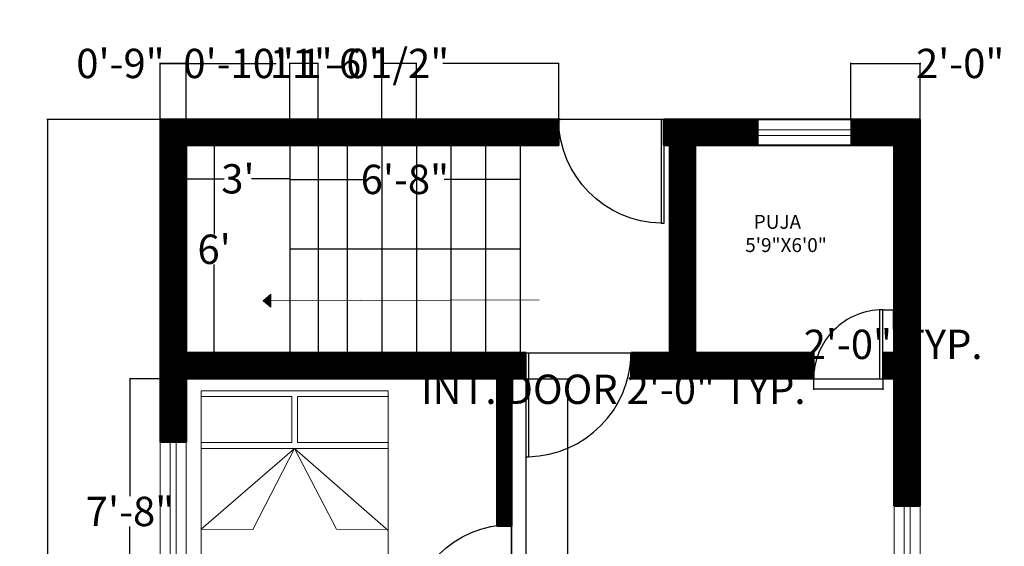
# Model space of a CAD drawing. Units: inches. Extents: x 254 to 1358, y 67 to 796.
# Tile 2 of 3: x 254 to 596, y 313 to 496. Entities that reach past the tile are written whole.
import ezdxf

# ---------------------------------------------------------------- set-up
doc = ezdxf.new("R2010")
doc.units = ezdxf.units.IN
doc.header["$MEASUREMENT"] = 0
for name, color, linetype, lineweight in [('A-ANNO-DIMS', 2, 'Continuous', 18), ('A-ANNO-SYMB', 7, 'Continuous', 18), ('A-AREA-IDEN', 7, 'Continuous', 18), ('A-FLOR-STRS', 7, 'Continuous', 25), ('A-FURN', 8, 'Continuous', 18), ('A-GLAZ', 160, 'Continuous', 18), ('A-WALL', 7, 'Continuous', 40), ('doors', 8, 'Continuous', 25)]:
    doc.layers.add(name, color=color, linetype=linetype, lineweight=lineweight)
doc.layers.add('A-ANNO-SYMB-PATT', color=251, linetype='Continuous', lineweight=13, true_color=0x636466)
doc.layers.add('A-WALL-PATT', color=251, linetype='Continuous', lineweight=13, true_color=0x636466)
doc.styles.get("Standard").update_dxf_attribs({"font": 'arial.ttf'})
doc.dimstyles.get("Standard").update_dxf_attribs({"dimtxt": 10.18, "dimasz": 0.18, "dimexe": 0.18, "dimexo": 0.0625, "dimgap": 0.09, "dimtad": 0, "dimtih": 1, "dimtoh": 1, "dimdec": 0, "dimzin": 0, "dimdsep": 46, "dimlunit": 3, "dimtxsty": 'Standard', "dimcen": 0.09, "dimadec": 0, "dimazin": 0, "dimtfac": 1, "dimtdec": 0, "dimtofl": 0, "dimtmove": 0, "dimatfit": 3, "dimfxl": 1, "dimtolj": 1, "dimtzin": 0, "dimarcsym": 0})

# ---------------------------------------------------------------- blocks, each defined once
blk = doc.blocks.new('*D1')
at = {"layer": 'A-ANNO-DIMS', "color": 0, "lineweight": -2, "transparency": 16777216}
for p, q in [((311.39, 452.48), (311.39, 440.81)), ((347.39, 452.48), (347.39, 440.81)), ((311.57, 440.99), (324.62, 440.99)), ((347.21, 440.99), (334.16, 440.99))]:
    blk.add_line(p, q, dxfattribs=at)
at = {"layer": 'A-ANNO-DIMS', "color": 0, "transparency": 16777216}
for points in [[(311.57, 441.02), (311.57, 440.96), (311.39, 440.99)], [(347.21, 441.02), (347.21, 440.96), (347.39, 440.99)]]:
    blk.add_solid(points, dxfattribs=at)
at = {"layer": 'Defpoints', "color": 0, "transparency": 16777216}
for p in [(311.39, 452.54), (347.39, 452.54), (347.39, 440.99)]:
    blk.add_point(p, dxfattribs=at)
at = {"layer": 'A-ANNO-DIMS', "color": 0, "transparency": 16777216, "insert": (329.39, 440.99), "char_height": 10.18, "attachment_point": 5}
blk.add_mtext("\\A1;3'", dxfattribs=at)
blk = doc.blocks.new('*D2')
at = {"layer": 'A-ANNO-DIMS', "color": 0, "lineweight": -2, "transparency": 16777216}
for p, q in [((347.39, 452.48), (347.39, 440.61)), ((427.39, 452.48), (427.39, 440.61)), ((347.57, 440.79), (373.74, 440.79)), ((427.21, 440.79), (401.04, 440.79))]:
    blk.add_line(p, q, dxfattribs=at)
at = {"layer": 'A-ANNO-DIMS', "color": 0, "transparency": 16777216}
for points in [[(347.57, 440.82), (347.57, 440.76), (347.39, 440.79)], [(427.21, 440.82), (427.21, 440.76), (427.39, 440.79)]]:
    blk.add_solid(points, dxfattribs=at)
at = {"layer": 'Defpoints', "color": 0, "transparency": 16777216}
for p in [(347.39, 452.54), (427.39, 452.54), (427.39, 440.79)]:
    blk.add_point(p, dxfattribs=at)
at = {"layer": 'A-ANNO-DIMS', "color": 0, "transparency": 16777216, "insert": (387.39, 440.79), "char_height": 10.18, "attachment_point": 5}
blk.add_mtext('\\A1;6\'-8"', dxfattribs=at)
blk = doc.blocks.new('*D3')
at = {"layer": 'A-ANNO-DIMS', "color": 0, "lineweight": -2, "transparency": 16777216}
for p, q in [((311.46, 452.54), (321.31, 452.54)), ((321.13, 452.36), (321.13, 421.83)), ((321.13, 380.72), (321.13, 411.26)), ((311.46, 380.54), (321.31, 380.54))]:
    blk.add_line(p, q, dxfattribs=at)
at = {"layer": 'A-ANNO-DIMS', "color": 0, "transparency": 16777216}
for points in [[(321.1, 452.36), (321.16, 452.36), (321.13, 452.54)], [(321.1, 380.72), (321.16, 380.72), (321.13, 380.54)]]:
    blk.add_solid(points, dxfattribs=at)
at = {"layer": 'Defpoints', "color": 0, "transparency": 16777216}
for p in [(311.39, 452.54), (311.39, 380.54), (321.13, 380.54)]:
    blk.add_point(p, dxfattribs=at)
at = {"layer": 'A-ANNO-DIMS', "color": 0, "transparency": 16777216, "insert": (321.13, 416.54), "char_height": 10.18, "attachment_point": 5}
blk.add_mtext("\\A1;6'", dxfattribs=at)
blk = doc.blocks.new('*D4')
at = {"layer": 'A-ANNO-DIMS', "color": 0, "lineweight": -2, "transparency": 16777216}
for p, q in [((302.33, 461.54), (263.04, 461.54)), ((263.22, 461.36), (263.22, 286.83)), ((263.22, 101.72), (263.22, 276.25)), ((302.33, 101.54), (263.04, 101.54))]:
    blk.add_line(p, q, dxfattribs=at)
at = {"layer": 'A-ANNO-DIMS', "color": 0, "transparency": 16777216}
for points in [[(263.19, 461.36), (263.25, 461.36), (263.22, 461.54)], [(263.19, 101.72), (263.25, 101.72), (263.22, 101.54)]]:
    blk.add_solid(points, dxfattribs=at)
at = {"layer": 'Defpoints', "color": 0, "transparency": 16777216}
for p in [(302.39, 461.54), (263.22, 101.54), (302.39, 101.54)]:
    blk.add_point(p, dxfattribs=at)
at = {"layer": 'A-ANNO-DIMS', "color": 0, "transparency": 16777216, "insert": (263.22, 281.54), "char_height": 10.18, "attachment_point": 5}
blk.add_mtext("\\A1;30'", dxfattribs=at)
blk = doc.blocks.new('WIN-48')
for p, q in [((9, 48), (0, 48)), ((0, 48), (0, 0)), ((3.5, 48), (3.5, 0)), ((5.5, 48), (5.5, 0)), ((5.5, 48), (5.5, 0)), ((5.5, 48), (5.5, 0)), ((5.5, 48), (5.5, 0)), ((9, 48), (9, 0)), ((9, 0), (0, 0))]:
    blk.add_line(p, q)
blk = doc.blocks.new('WIN-32')
for p, q in [((0, 0), (0, 9)), ((32.11, 9), (0, 9)), ((32.11, 0), (32.11, 9)), ((32.11, 5.5), (0, 5.5)), ((32.11, 3.5), (0, 3.5)), ((32.11, 3.5), (0, 3.5)), ((32.11, 3.5), (0, 3.5)), ((32.11, 3.5), (0, 3.5)), ((32.11, 0), (0, 0))]:
    blk.add_line(p, q)
blk = doc.blocks.new('DOOR-SWING-36')
for p, q in [((0, 0), (-36, 0)), ((-36, 0), (-36, -1)), ((0, 0), (0, -36.57)), ((0, -1), (-36, -1))]:
    blk.add_line(p, q)
blk.add_arc((0.31, -0.26), 36.31, 181.1696, 269.5155)
blk = doc.blocks.new('DOOR-SWING-24-INT')
for p, q in [((24, 0), (0, 0)), ((0, 0), (0, -24)), ((1, 0), (1, -24))]:
    blk.add_line(p, q)
blk.add_arc((0.03, -0.01), 23.97, 269.9169, 0.0334)
blk = doc.blocks.new('BED-DOUBLE')
for p, q in [((65, 72), (0, 72)), ((0, 72), (0, 0)), ((65, 0), (65, 72)), ((0, 48.04), (18, 48.19)), ((32.5, 20), (0, 48.04)), ((32.5, 20), (18, 48.19)), ((32.5, 20), (65, 48.44)), ((47, 48.04), (32.5, 20)), ((47, 48.04), (65, 48.19)), ((0, 20), (65, 20)), ((0, 18), (31.5, 18)), ((31.5, 18), (31.5, 2)), ((33.5, 18), (33.5, 2)), ((33.5, 18), (65, 18)), ((0, 2), (31.5, 2)), ((0, 0), (65, 0)), ((33.5, 2), (65, 2))]:
    blk.add_line(p, q)
blk = doc.blocks.new('*D28')
at = {"layer": 'A-ANNO-DIMS', "color": 0, "lineweight": -2, "transparency": 16777216}
for p, q in [((529.39, 371.48), (529.39, 367.76)), ((553.39, 371.48), (553.39, 367.76)), ((529.39, 367.94), (529.21, 367.94)), ((553.21, 367.94), (529.57, 367.94))]:
    blk.add_line(p, q, dxfattribs=at)
at = {"layer": 'A-ANNO-DIMS', "color": 0, "transparency": 16777216}
for points in [[(529.57, 367.97), (529.57, 367.91), (529.39, 367.94)], [(553.21, 367.97), (553.21, 367.91), (553.39, 367.94)]]:
    blk.add_solid(points, dxfattribs=at)
at = {"layer": 'Defpoints', "color": 0, "transparency": 16777216}
for p in [(529.39, 371.54), (553.39, 371.54), (529.39, 367.94)]:
    blk.add_point(p, dxfattribs=at)
at = {"layer": 'A-ANNO-DIMS', "color": 0, "transparency": 16777216, "insert": (459.75, 367.94), "char_height": 10.18, "attachment_point": 5}
blk.add_mtext('\\A1;INT. DOOR 2\'-0" TYP.', dxfattribs=at)
blk = doc.blocks.new('*D29')
at = {"layer": 'A-ANNO-DIMS', "color": 0, "lineweight": -2, "transparency": 16777216}
for p, q in [((553.46, 395.54), (557.17, 395.54)), ((556.99, 395.36), (556.99, 388.83)), ((556.99, 371.72), (556.99, 378.26)), ((553.46, 371.54), (557.17, 371.54))]:
    blk.add_line(p, q, dxfattribs=at)
at = {"layer": 'A-ANNO-DIMS', "color": 0, "transparency": 16777216}
for points in [[(556.96, 395.36), (557.02, 395.36), (556.99, 395.54)], [(556.96, 371.72), (557.02, 371.72), (556.99, 371.54)]]:
    blk.add_solid(points, dxfattribs=at)
at = {"layer": 'Defpoints', "color": 0, "transparency": 16777216}
for p in [(553.39, 395.54), (553.39, 371.54), (556.99, 371.54)]:
    blk.add_point(p, dxfattribs=at)
at = {"layer": 'A-ANNO-DIMS', "color": 0, "transparency": 16777216, "insert": (556.99, 383.54), "char_height": 10.18, "attachment_point": 5}
blk.add_mtext('\\A1;2\'-0" TYP.', dxfattribs=at)
blk = doc.blocks.new('*D41')
at = {"layer": 'A-ANNO-DIMS', "color": 0, "lineweight": -2, "transparency": 16777216}
for p, q in [((302.39, 461.61), (302.39, 481.21)), ((302.57, 481.03), (342.65, 481.03)), ((440.64, 481.03), (400.56, 481.03)), ((440.82, 461.6), (440.82, 481.21))]:
    blk.add_line(p, q, dxfattribs=at)
at = {"layer": 'A-ANNO-DIMS', "color": 0, "transparency": 16777216}
for points in [[(302.57, 481.06), (302.57, 481), (302.39, 481.03)], [(440.64, 481.06), (440.64, 481), (440.82, 481.03)]]:
    blk.add_solid(points, dxfattribs=at)
at = {"layer": 'Defpoints', "color": 0, "transparency": 16777216}
for p in [(440.82, 481.03), (302.39, 461.54), (440.82, 461.54)]:
    blk.add_point(p, dxfattribs=at)
at = {"layer": 'A-ANNO-DIMS', "color": 0, "transparency": 16777216, "insert": (371.61, 481.03), "char_height": 10.18, "attachment_point": 5}
blk.add_mtext('\\A1;11\'-6 1/2"', dxfattribs=at)
blk = doc.blocks.new('*D42')
at = {"layer": 'A-ANNO-DIMS', "color": 0, "lineweight": -2, "transparency": 16777216}
for p, q in [((542.27, 461.61), (542.27, 481.21)), ((542.45, 481.03), (566.21, 481.03)), ((566.39, 461.61), (566.39, 481.21)), ((566.39, 481.03), (566.57, 481.03))]:
    blk.add_line(p, q, dxfattribs=at)
at = {"layer": 'A-ANNO-DIMS', "color": 0, "transparency": 16777216}
for points in [[(542.45, 481.06), (542.45, 481), (542.27, 481.03)], [(566.21, 481.06), (566.21, 481), (566.39, 481.03)]]:
    blk.add_solid(points, dxfattribs=at)
at = {"layer": 'Defpoints', "color": 0, "transparency": 16777216}
for p in [(566.39, 481.03), (542.27, 461.54), (566.39, 461.54)]:
    blk.add_point(p, dxfattribs=at)
at = {"layer": 'A-ANNO-DIMS', "color": 0, "transparency": 16777216, "insert": (580.28, 481.03), "char_height": 10.18, "attachment_point": 5}
blk.add_mtext('\\A1;2\'-0"', dxfattribs=at)
blk = doc.blocks.new('*D45')
at = {"layer": 'A-ANNO-DIMS', "color": 0, "lineweight": -2, "transparency": 16777216}
for p, q in [((302.39, 481.03), (302.21, 481.03)), ((302.39, 461.61), (302.39, 481.21)), ((311.21, 481.03), (302.57, 481.03)), ((311.39, 452.61), (311.39, 481.21))]:
    blk.add_line(p, q, dxfattribs=at)
at = {"layer": 'A-ANNO-DIMS', "color": 0, "transparency": 16777216}
for points in [[(302.57, 481.06), (302.57, 481), (302.39, 481.03)], [(311.21, 481.06), (311.21, 481), (311.39, 481.03)]]:
    blk.add_solid(points, dxfattribs=at)
at = {"layer": 'Defpoints', "color": 0, "transparency": 16777216}
for p in [(302.39, 481.03), (302.39, 461.54), (311.39, 452.54)]:
    blk.add_point(p, dxfattribs=at)
at = {"layer": 'A-ANNO-DIMS', "color": 0, "transparency": 16777216, "insert": (288.59, 481.03), "char_height": 10.18, "attachment_point": 5}
blk.add_mtext('\\A1;0\'-9"', dxfattribs=at)
blk = doc.blocks.new('*D47')
at = {"layer": 'A-ANNO-DIMS', "color": 0, "lineweight": -2, "transparency": 16777216}
for p, q in [((311.33, 371.54), (291.72, 371.54)), ((291.9, 371.36), (291.9, 330.83)), ((291.9, 279.72), (291.9, 320.26)), ((311.33, 279.54), (291.72, 279.54))]:
    blk.add_line(p, q, dxfattribs=at)
at = {"layer": 'A-ANNO-DIMS', "color": 0, "transparency": 16777216}
for points in [[(291.87, 371.36), (291.93, 371.36), (291.9, 371.54)], [(291.87, 279.72), (291.93, 279.72), (291.9, 279.54)]]:
    blk.add_solid(points, dxfattribs=at)
at = {"layer": 'Defpoints', "color": 0, "transparency": 16777216}
for p in [(291.9, 371.54), (311.39, 371.54), (311.39, 279.54)]:
    blk.add_point(p, dxfattribs=at)
at = {"layer": 'A-ANNO-DIMS', "color": 0, "transparency": 16777216, "insert": (291.9, 325.54), "char_height": 10.18, "attachment_point": 5}
blk.add_mtext('\\A1;7\'-8"', dxfattribs=at)
blk = doc.blocks.new('*D49')
at = {"layer": 'A-ANNO-DIMS', "color": 0, "lineweight": -2, "transparency": 16777216}
for p, q in [((424.46, 371.54), (444.06, 371.54)), ((443.88, 371.36), (443.88, 308.74)), ((443.88, 235.72), (443.88, 298.34)), ((424.46, 235.54), (444.06, 235.54))]:
    blk.add_line(p, q, dxfattribs=at)
at = {"layer": 'A-ANNO-DIMS', "color": 0, "transparency": 16777216}
for points in [[(443.85, 371.36), (443.91, 371.36), (443.88, 371.54)], [(443.85, 235.72), (443.91, 235.72), (443.88, 235.54)]]:
    blk.add_solid(points, dxfattribs=at)
at = {"layer": 'Defpoints', "color": 0, "transparency": 16777216}
for p in [(424.39, 371.54), (424.39, 235.54), (443.88, 235.54)]:
    blk.add_point(p, dxfattribs=at)
at = {"layer": 'A-ANNO-DIMS', "color": 0, "transparency": 16777216, "insert": (443.88, 303.54), "char_height": 10.18, "attachment_point": 5}
blk.add_mtext('\\A1;11\'-4"', dxfattribs=at)
blk = doc.blocks.new('*D54')
at = {"layer": 'A-ANNO-DIMS', "color": 0, "lineweight": -2, "transparency": 16777216}
for p, q in [((347.39, 481.03), (347.21, 481.03)), ((347.39, 452.61), (347.39, 481.21)), ((357.12, 481.03), (347.57, 481.03)), ((357.3, 452.61), (357.3, 481.21))]:
    blk.add_line(p, q, dxfattribs=at)
at = {"layer": 'A-ANNO-DIMS', "color": 0, "transparency": 16777216}
for points in [[(347.57, 481.06), (347.57, 481), (347.39, 481.03)], [(357.12, 481.06), (357.12, 481), (357.3, 481.03)]]:
    blk.add_solid(points, dxfattribs=at)
at = {"layer": 'Defpoints', "color": 0, "transparency": 16777216}
for p in [(347.39, 481.03), (347.39, 452.54), (357.3, 452.54)]:
    blk.add_point(p, dxfattribs=at)
at = {"layer": 'A-ANNO-DIMS', "color": 0, "transparency": 16777216, "insert": (329.64, 481.03), "char_height": 10.18, "attachment_point": 5}
blk.add_mtext('\\A1;0\'-10"', dxfattribs=at)
blk = doc.blocks.new('*D55')
at = {"layer": 'A-ANNO-DIMS', "color": 0, "lineweight": -2, "transparency": 16777216}
for p, q in [((379.39, 481.03), (379.21, 481.03)), ((379.39, 452.61), (379.39, 481.21)), ((391.21, 481.03), (379.57, 481.03)), ((391.39, 452.61), (391.39, 481.21))]:
    blk.add_line(p, q, dxfattribs=at)
at = {"layer": 'A-ANNO-DIMS', "color": 0, "transparency": 16777216}
for points in [[(379.57, 481.06), (379.57, 481), (379.39, 481.03)], [(391.21, 481.06), (391.21, 481), (391.39, 481.03)]]:
    blk.add_solid(points, dxfattribs=at)
at = {"layer": 'Defpoints', "color": 0, "transparency": 16777216}
for p in [(379.39, 481.03), (379.39, 452.54), (391.39, 452.54)]:
    blk.add_point(p, dxfattribs=at)
at = {"layer": 'A-ANNO-DIMS', "color": 0, "transparency": 16777216, "insert": (366.07, 481.03), "char_height": 10.18, "attachment_point": 5}
blk.add_mtext('\\A1;1\'-0"', dxfattribs=at)
blk = doc.blocks.new('*D56')
at = {"layer": 'A-ANNO-DIMS', "color": 0, "lineweight": -2, "transparency": 16777216}
for p, q in [((429.39, 380.48), (429.39, 81.87)), ((424.39, 371.48), (424.39, 81.87)), ((424.57, 82.05), (429.21, 82.05)), ((429.39, 82.05), (429.57, 82.05))]:
    blk.add_line(p, q, dxfattribs=at)
at = {"layer": 'A-ANNO-DIMS', "color": 0, "transparency": 16777216}
for points in [[(424.57, 82.08), (424.57, 82.02), (424.39, 82.05)], [(429.21, 82.08), (429.21, 82.02), (429.39, 82.05)]]:
    blk.add_solid(points, dxfattribs=at)
at = {"layer": 'Defpoints', "color": 0, "transparency": 16777216}
for p in [(429.39, 380.54), (424.39, 371.54), (429.39, 82.05)]:
    blk.add_point(p, dxfattribs=at)
at = {"layer": 'A-ANNO-DIMS', "color": 0, "transparency": 16777216, "insert": (443.19, 82.05), "char_height": 10.18, "attachment_point": 5}
blk.add_mtext('\\A1;0\'-5"', dxfattribs=at)

msp = doc.modelspace()

# ---------------------------------------------------------------- hatches: boundary and pattern name
at = {"layer": 'A-ANNO-SYMB-PATT'}
h = msp.add_hatch(dxfattribs=at)
h.set_pattern_fill('ANSI31', color=256)
h.paths.add_polyline_path([(340.85, 400.97), (338.14, 398.67), (340.86, 396.39), (340.85, 398.68)])
at = {"layer": 'A-WALL-PATT'}
h = msp.add_hatch(dxfattribs=at)
h.set_pattern_fill('ANSI31', color=256)
h.paths.add_polyline_path([(311.39, 452.54), (440.82, 452.54), (440.82, 461.54), (440.82, 461.54), (302.39, 461.54), (302.39, 349.54), (311.39, 349.54), (311.39, 371.54), (419.39, 371.54), (419.39, 320.73, -0.034566), (424.39, 321.12), (424.39, 371.54), (429.39, 371.54), (429.39, 380.54), (311.39, 380.54)])
h.paths.add_polyline_path([(424.39, 284.54), (419.39, 284.54), (419.39, 279.54), (311.39, 279.54), (311.39, 301.54), (302.39, 301.54), (302.39, 263.04), (311.39, 263.04), (311.39, 274.54), (395.39, 274.54), (395.39, 264.04), (400.39, 264.04), (400.39, 274.54), (424.39, 274.54)])
h.paths.add_polyline_path([(311.39, 230.54), (419.39, 230.54), (419.39, 225.54), (424.39, 225.54), (424.39, 235.54), (400.39, 235.54), (400.39, 240.04), (395.39, 240.04), (395.39, 235.54), (311.39, 235.54), (311.39, 247.04), (302.39, 247.04), (302.39, 186.84), (311.39, 186.84)])
h.paths.add_polyline_path([(311.39, 138.84), (302.39, 138.84), (302.39, 101.54), (435.39, 101.54), (435.39, 110.54), (424.39, 110.54), (424.39, 173.54), (429.39, 173.54), (429.39, 178.54), (424.39, 178.54), (424.39, 188.97, -0.034564), (419.39, 189.35), (419.39, 110.54), (311.39, 110.54)])
h.paths.add_polyline_path([(510.16, 461.54), (477.39, 461.54), (477.39, 452.54), (479.39, 452.54), (479.39, 380.54), (465.96, 380.54), (465.96, 371.54), (529.39, 371.54), (529.39, 380.54), (488.39, 380.54), (488.39, 452.54), (510.16, 452.54)])
h.paths.add_polyline_path([(566.39, 461.54), (542.27, 461.54), (542.27, 452.54), (557.39, 452.54), (557.39, 380.54), (553.39, 380.54), (553.39, 371.54), (557.39, 371.54), (557.39, 327.54), (566.39, 327.54)])
h.paths.add_polyline_path([(566.39, 279.54), (557.39, 279.54), (557.39, 235.54), (467.39, 235.54), (467.39, 230.54), (557.39, 230.54), (557.39, 194.54), (566.39, 194.54)])
h.paths.add_polyline_path([(566.39, 146.54), (557.39, 146.54), (557.39, 110.54), (495.53, 110.54), (495.53, 101.54), (566.39, 101.54)])
h.paths.add_polyline_path([(479.53, 110.54), (467.39, 110.54), (467.39, 178.54), (453.39, 178.54), (453.39, 173.54), (462.39, 173.54), (462.39, 110.54), (451.39, 110.54), (451.39, 101.54), (479.53, 101.54)])

# ---------------------------------------------------------------- linework, layer by layer
at = {"layer": 'A-ANNO-SYMB'}
for p, q in [((340.85, 400.97), (338.14, 398.67)), ((340.85, 398.68), (340.85, 400.97)), ((338.14, 398.67), (340.86, 396.39)), ((434.09, 398.97), (340.85, 398.68)), ((340.86, 396.39), (340.85, 398.68))]:
    msp.add_line(p, q, dxfattribs=at)
at = {"layer": 'A-FLOR-STRS'}
for p, q in [((347.39, 452.54), (347.39, 380.54)), ((357.3, 452.54), (357.3, 380.54)), ((367.39, 452.54), (367.39, 380.54)), ((379.39, 452.54), (379.39, 380.54)), ((379.39, 452.54), (379.39, 380.54)), ((391.39, 452.54), (391.39, 380.54)), ((403.39, 452.54), (403.39, 380.54)), ((415.39, 452.54), (415.39, 380.54)), ((427.39, 452.54), (427.39, 380.54)), ((427.39, 416.54), (347.39, 416.54))]:
    msp.add_line(p, q, dxfattribs=at)
at = {"layer": 'A-WALL'}
for p, q in [((302.39, 461.54), (302.39, 349.54)), ((441.39, 461.54), (302.39, 461.54)), ((440.82, 452.54), (440.82, 461.54)), ((566.39, 461.54), (477.39, 461.54)), ((477.39, 452.54), (477.39, 461.54)), ((566.39, 327.54), (566.39, 461.54)), ((311.39, 452.54), (311.39, 380.54)), ((440.82, 452.54), (311.39, 452.54)), ((479.39, 452.54), (477.39, 452.54)), ((479.39, 380.54), (479.39, 452.54)), ((557.39, 452.54), (488.39, 452.54)), ((488.39, 380.54), (488.39, 452.54)), ((557.39, 380.54), (557.39, 452.54)), ((429.39, 380.54), (311.39, 380.54)), ((429.39, 371.54), (429.39, 380.54)), ((479.39, 380.54), (465.96, 380.54)), ((465.96, 371.54), (465.96, 380.54)), ((529.39, 380.54), (488.39, 380.54)), ((529.39, 380.54), (529.39, 371.54)), ((557.39, 380.54), (553.39, 380.54)), ((553.39, 380.54), (553.39, 371.54)), ((311.39, 371.54), (311.39, 349.54)), ((419.39, 371.54), (311.39, 371.54)), ((419.39, 371.54), (419.39, 320.54)), ((424.39, 371.54), (424.39, 320.54)), ((429.39, 371.54), (424.39, 371.54)), ((529.39, 371.54), (465.96, 371.54)), ((557.39, 371.54), (553.39, 371.54)), ((557.39, 327.54), (557.39, 371.54)), ((311.39, 349.54), (302.39, 349.54)), ((557.39, 327.54), (566.39, 327.54)), ((419.39, 320.54), (424.39, 320.54))]:
    msp.add_line(p, q, dxfattribs=at)

# ---------------------------------------------------------------- block references
at = {"layer": 'A-FURN', "extrusion": (0, 0, -1), "zscale": -1, "rotation": 180}
msp.add_blockref('BED-DOUBLE', (-316.59, 367.42), dxfattribs=at)
at = {"layer": 'A-GLAZ'}
for name, p in [('WIN-32', (510.16, 452.54)), ('WIN-48', (302.39, 301.54)), ('WIN-48', (557.39, 279.54))]:
    msp.add_blockref(name, p, dxfattribs=at)
at = {"layer": 'doors', "extrusion": (0, 0, -1), "zscale": -1}
for p, rotation in [((-477.39, 461.54), 89.99999999999982), ((-424.39, 284.54), 180)]:
    msp.add_blockref('DOOR-SWING-36', p, dxfattribs=dict(at, rotation=rotation))
at = {"layer": 'doors'}
for name, p, rotation in [('DOOR-SWING-24-INT', (553.39, 371.54), 180), ('DOOR-SWING-36', (429.39, 380.54), 90.00000000000017)]:
    msp.add_blockref(name, p, dxfattribs=dict(at, rotation=rotation))

# ---------------------------------------------------------------- texts
at = {"layer": 'A-AREA-IDEN', "insert": (505.61, 428.47), "char_height": 4.835, "attachment_point": 1}
msp.add_mtext_dynamic_manual_height_columns('  PUJA \\P5\'9"X6\'0"', width=48.103, gutter_width=24.18, heights=[18.78], dxfattribs=at)

# ---------------------------------------------------------------- dimensions: what is measured, and where the dimension line sits
at = {"layer": 'A-ANNO-DIMS'}
for base, p1, p2, override, picture, middle in [((440.82, 481.03), (302.39, 461.54), (440.82, 461.54), {"dimdec": 1, "dimlfac": 1, "dimrnd": 0, "dimzin": 1, "dimdsep": 46, "dimlunit": 4, "dimfrac": 2}, '*D41', (371.61, 481.03)), ((302.39, 481.03), (311.39, 452.54), (302.39, 461.54), {"dimdec": 1, "dimlfac": 1, "dimrnd": 0, "dimzin": 1, "dimdsep": 46, "dimlunit": 4, "dimfrac": 2}, '*D45', (288.59, 481.03)), ((347.39, 481.03), (357.3, 452.54), (347.39, 452.54), {"dimdec": 1, "dimlfac": 1, "dimrnd": 0, "dimzin": 1, "dimdsep": 46, "dimlunit": 4, "dimfrac": 2}, '*D54', (329.64, 481.03)), ((379.39, 481.03), (391.39, 452.54), (379.39, 452.54), {"dimdec": 1, "dimlfac": 1, "dimrnd": 0, "dimzin": 1, "dimdsep": 46, "dimlunit": 4, "dimfrac": 2}, '*D55', (366.07, 481.03)), ((566.39, 481.03), (542.27, 461.54), (566.39, 461.54), {"dimdec": 1, "dimlfac": 1, "dimrnd": 0, "dimzin": 1, "dimdsep": 46, "dimlunit": 4, "dimfrac": 2}, '*D42', (580.28, 481.03)), ((347.39, 440.99), (311.39, 452.54), (347.39, 452.54), {"dimclrd": 0, "dimclre": 0, "dimclrt": 0}, '*D1', (329.39, 440.99)), ((427.39, 440.79), (347.39, 452.54), (427.39, 452.54), {"dimclrd": 0, "dimclre": 0, "dimclrt": 0}, '*D2', (387.39, 440.79)), ((429.39, 82.05), (424.39, 371.54), (429.39, 380.54), {"dimdec": 1, "dimlfac": 1, "dimrnd": 0, "dimzin": 1, "dimdsep": 46, "dimlunit": 4, "dimfrac": 2}, '*D56', (443.19, 82.05))]:
    dim = msp.add_linear_dim(base=base, p1=p1, p2=p2, dimstyle='Standard', override=override, dxfattribs=at)
    dim.commit()
    dim.dimension.update_dxf_attribs({"geometry": picture, "text_midpoint": middle})
for base, p1, p2, angle, override, picture, middle in [((263.22, 101.54), (302.39, 461.54), (302.39, 101.54), 90, {"dimclrd": 0, "dimclre": 0, "dimclrt": 0}, '*D4', (263.22, 281.54)), ((321.13, 380.54), (311.39, 452.54), (311.39, 380.54), 90, {"dimclrd": 0, "dimclre": 0, "dimclrt": 0}, '*D3', (321.13, 416.54)), ((291.9, 371.54), (311.39, 279.54), (311.39, 371.54), 90, {"dimdec": 1, "dimlfac": 1, "dimrnd": 0, "dimzin": 1, "dimdsep": 46, "dimlunit": 4, "dimfrac": 2}, '*D47', (291.9, 325.54)), ((443.88, 235.54), (424.39, 371.54), (424.39, 235.54), 270, {"dimdec": 1, "dimlfac": 1, "dimrnd": 0, "dimzin": 1, "dimdsep": 46, "dimlunit": 4, "dimfrac": 2}, '*D49', (443.88, 303.54))]:
    dim = msp.add_linear_dim(base=base, p1=p1, p2=p2, angle=angle, dimstyle='Standard', override=override, dxfattribs=at)
    dim.commit()
    dim.dimension.update_dxf_attribs({"geometry": picture, "text_midpoint": middle})
for base, p1, p2, angle, text, picture, middle in [((529.39, 367.94), (553.39, 371.54), (529.39, 371.54), 180, 'INT. DOOR <> TYP.', '*D28', (459.75, 367.94)), ((556.99, 371.54), (553.39, 395.54), (553.39, 371.54), 270, '<> TYP.', '*D29', (556.99, 383.54))]:
    dim = msp.add_linear_dim(base=base, p1=p1, p2=p2, angle=angle, text=text, dimstyle='Standard', override={"dimdec": 1, "dimlfac": 1, "dimrnd": 0, "dimzin": 1, "dimdsep": 46, "dimlunit": 4, "dimfrac": 2}, dxfattribs=at)
    dim.commit()
    dim.dimension.update_dxf_attribs({"geometry": picture, "text_midpoint": middle})

doc.saveas('drawing.dxf')
